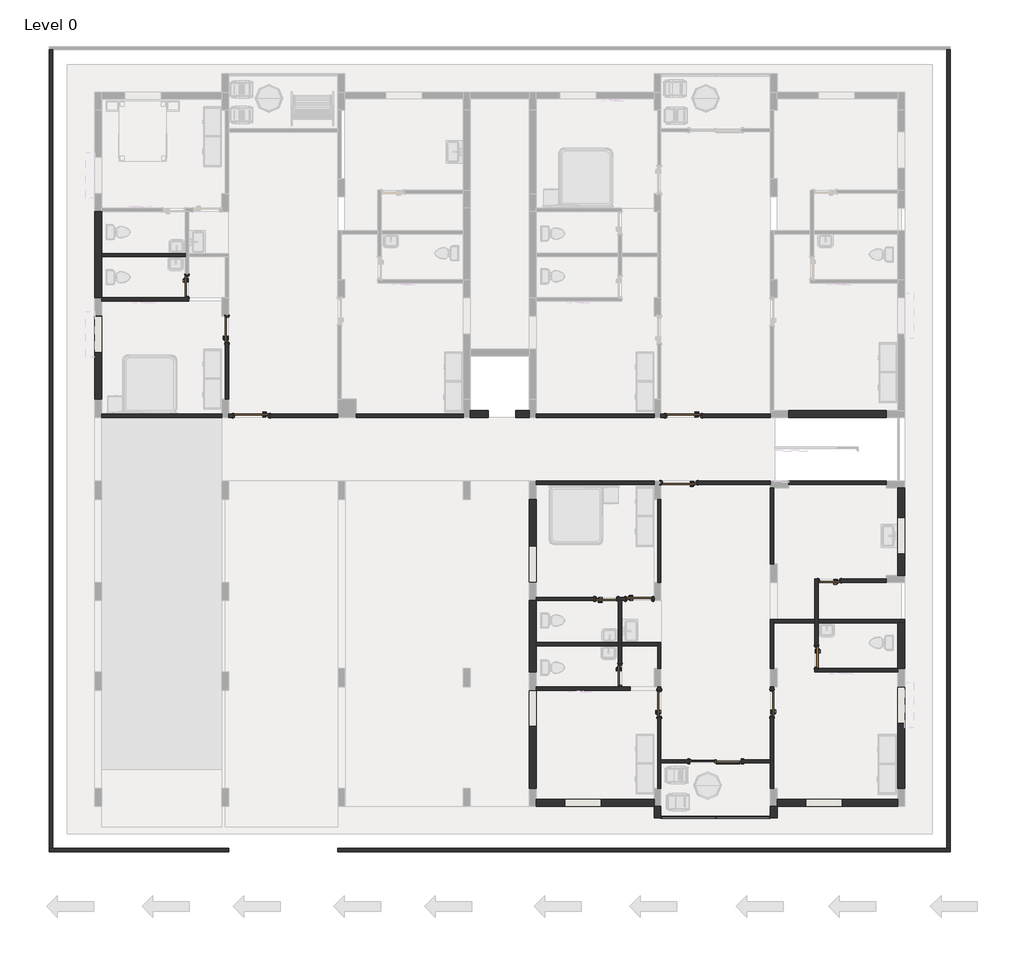
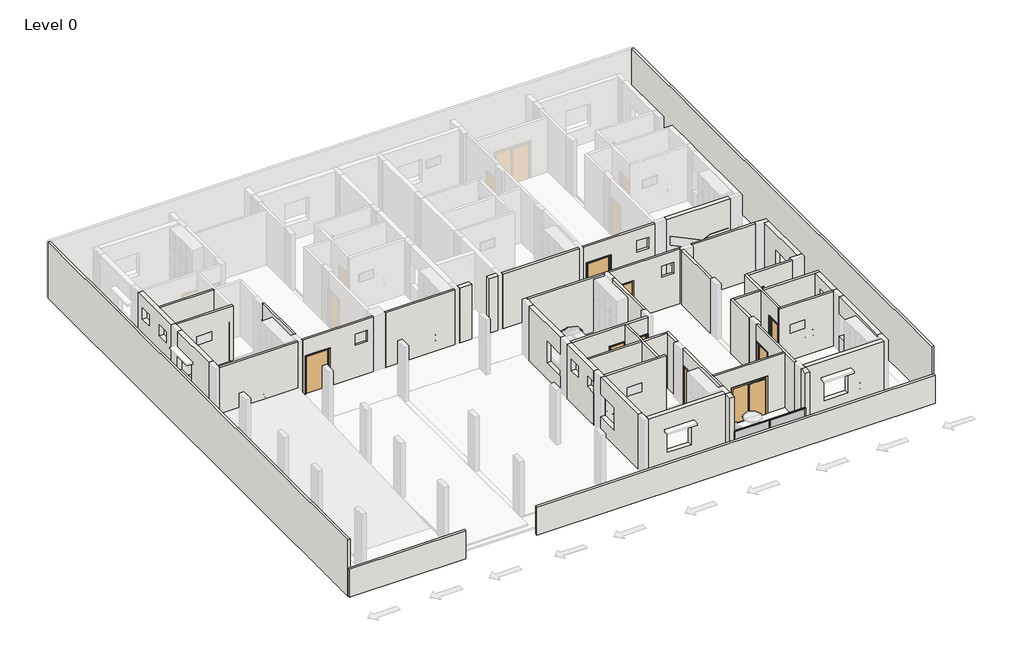
# One storey, part 1 of 6: 46 walls, 13 doors, 5 members, 2 plates.
"""IFC4 building model written with IfcOpenShell, lengths in millimetres."""

from ifc_helpers import new_model, si_unit, frame, origin, origin_with_axes, place, context, project, spatial, polyline, outline, extrude, faceted_brep, transform, mapped, element, save
from components import door_c5e969d5, door_d225582b, door_4bb05ab8, doors_intsgl_3_11801b65, doors_intsgl_3_f3216364, doors_intsgl_4_41b074ad, doors_intsgl_4_134d4d27, rectangular_mullion_30mm_square_b78902bc, rectangular_mullion_30mm_square_f98953c9, rectangular_mullion_30mm_square_8997babb, rectangular_mullion_30mm_square_5c6859bd, system_panel_glazed_e8634194, system_panel_glazed_30ab8f14

model = new_model("IFC4")

# Units and contexts
model_context = context("Model", 3, world=origin())
ifc_project = project(units=[si_unit("LENGTHUNIT", "METRE", prefix="MILLI")], contexts=[model_context])

# Site, building, storey
site = spatial("IfcSite", under=ifc_project)
building = spatial("IfcBuilding", under=site)
storey = spatial("IfcBuildingStorey", under=building, Name="Level 0", Elevation=0.0)

# Doors
placement = place(None, origin())
door_shape = door_c5e969d5(model_context)
element("IfcDoor", 1, ObjectType="Door-Double-Sliding : 5'8\"", at=placement, inside=storey, context=model_context, shape_type="MappedRepresentation", body=[
    mapped(door_shape, transform((7286.1098461, -11905.3017861, 0.0), x_axis=(-1.0, 0.0, 0.0), y_axis=(0.0, -1.0, 0.0), z_axis=(0.0, 0.0, 1.0))),
])
door_2_shape = door_d225582b(model_context)
element("IfcDoor", 2, ObjectType="Doors_IntSgl : 2'6\"", at=placement, inside=storey, context=model_context, shape_type="MappedRepresentation", body=[
    mapped(door_2_shape, transform((-10393.0197227, 3860.6022446, 0.0), x_axis=(0.0, -1.0, 0.0), y_axis=(1.0, 0.0, 0.0), z_axis=(0.0, 0.0, 1.0))),
])
element("IfcDoor", 3, ObjectType="Doors_IntSgl : 2'6\"", at=placement, inside=storey, context=model_context, shape_type="MappedRepresentation", body=[
    mapped(door_2_shape, transform((4085.7098461, -9155.7517861, 0.0), x_axis=(0.0, -1.0, 0.0), y_axis=(1.0, 0.0, 0.0), z_axis=(0.0, 0.0, 1.0))),
])
element("IfcDoor", 4, ObjectType="Doors_IntSgl : 2'6\"", at=placement, inside=storey, context=model_context, shape_type="MappedRepresentation", body=[
    mapped(door_2_shape, transform((3634.8598461, -6596.7017861, 0.0), x_axis=(1.0, 0.0, 0.0), y_axis=(0.0, 1.0, 0.0), z_axis=(0.0, 0.0, 1.0))),
])
door_3_shape = door_4bb05ab8(model_context)
element("IfcDoor", 5, ObjectType="Doors_IntSgl : 2'6\"", at=placement, inside=storey, context=model_context, shape_type="MappedRepresentation", body=[
    mapped(door_3_shape, transform((11096.1098461, -5987.1017861, 0.0), x_axis=(-1.0, 0.0, 0.0), y_axis=(0.0, -1.0, 0.0), z_axis=(0.0, 0.0, 1.0))),
])
element("IfcDoor", 6, ObjectType="Doors_IntSgl : 2'6\"", at=placement, inside=storey, context=model_context, shape_type="MappedRepresentation", body=[
    mapped(door_3_shape, transform((10657.9598461, -8546.1517861, 0.0), x_axis=(0.0, -1.0, 0.0), y_axis=(1.0, 0.0, 0.0), z_axis=(0.0, 0.0, 1.0))),
])
doors_intsgl_3_shape = doors_intsgl_3_11801b65(model_context)
element("IfcDoor", 7, ObjectType="Doors_IntSgl : 3'", at=placement, inside=storey, context=model_context, shape_type="MappedRepresentation", body=[
    mapped(doors_intsgl_3_shape, transform((-9058.7901539, 2413.9482139, 0.0), x_axis=(0.0, 1.0, 0.0), y_axis=(-1.0, 0.0, 0.0), z_axis=(0.0, 0.0, 1.0))),
])
element("IfcDoor", 8, ObjectType="Doors_IntSgl : 3'", at=placement, inside=storey, context=model_context, shape_type="MappedRepresentation", body=[
    mapped(doors_intsgl_3_shape, transform((5400.1598461, -10108.2517861, 0.0), x_axis=(0.0, 1.0, 0.0), y_axis=(-1.0, 0.0, 0.0), z_axis=(0.0, 0.0, 1.0))),
])
element("IfcDoor", 9, ObjectType="Doors_IntSgl : 3'", at=placement, inside=storey, context=model_context, shape_type="MappedRepresentation", body=[
    mapped(doors_intsgl_3_shape, transform((4733.4098461, -6596.7017861, 0.0), x_axis=(1.0, 0.0, 0.0), y_axis=(0.0, 1.0, 0.0), z_axis=(0.0, 0.0, 1.0))),
])
doors_intsgl_3_2_shape = doors_intsgl_3_f3216364(model_context)
element("IfcDoor", 10, ObjectType="Doors_IntSgl : 3'", at=placement, inside=storey, context=model_context, shape_type="MappedRepresentation", body=[
    mapped(doors_intsgl_3_2_shape, transform((9172.0598461, -10095.5517861, 0.0), x_axis=(0.0, 1.0, 0.0), y_axis=(-1.0, 0.0, 0.0), z_axis=(0.0, 0.0, 1.0))),
])
doors_intsgl_4_shape = doors_intsgl_4_41b074ad(model_context)
element("IfcDoor", 11, ObjectType="Doors_IntSgl : 4'", at=placement, inside=storey, context=model_context, shape_type="MappedRepresentation", body=[
    mapped(doors_intsgl_4_shape, transform((-8239.6401539, -463.7477554, 0.0), x_axis=(-1.0, 0.0, 0.0), y_axis=(0.0, -1.0, 0.0), z_axis=(0.0, 0.0, 1.0))),
])
element("IfcDoor", 12, ObjectType="Doors_IntSgl : 4'", at=placement, inside=storey, context=model_context, shape_type="MappedRepresentation", body=[
    mapped(doors_intsgl_4_shape, transform((6219.3098461, -462.6017861, 0.0), x_axis=(-1.0, 0.0, 0.0), y_axis=(0.0, -1.0, 0.0), z_axis=(0.0, 0.0, 1.0))),
])
doors_intsgl_4_2_shape = doors_intsgl_4_134d4d27(model_context)
element("IfcDoor", 13, ObjectType="Doors_IntSgl : 4'", at=placement, inside=storey, context=model_context, shape_type="MappedRepresentation", body=[
    mapped(doors_intsgl_4_2_shape, transform((6066.9098461, -2710.5017861, 0.0), x_axis=(-1.0, 0.0, 0.0), y_axis=(0.0, -1.0, 0.0), z_axis=(0.0, 0.0, 1.0))),
])

# Members
rectangular_mullion_30mm_square_shape = rectangular_mullion_30mm_square_b78902bc(model_context)
element("IfcMember", 14, ObjectType="Rectangular Mullion : 30mm_Square", at=placement, inside=storey, context=model_context, shape_type="MappedRepresentation", body=[
    mapped(rectangular_mullion_30mm_square_shape, transform((7272.9093803, -13918.2517861, 1164.8147652), x_axis=(0.0, 0.0, 1.0), y_axis=(0.0, -1.0, 0.0), z_axis=(1.0, 0.0, 0.0))),
])
rectangular_mullion_30mm_square_2_shape = rectangular_mullion_30mm_square_f98953c9(model_context)
element("IfcMember", 15, ObjectType="Rectangular Mullion : 30mm_Square", at=placement, inside=storey, context=model_context, shape_type="MappedRepresentation", body=[
    mapped(rectangular_mullion_30mm_square_2_shape, transform((9114.9098461, -13918.2517861, 98.0147652), x_axis=(1.0, 0.0, 0.0), y_axis=(0.0, -1.0, 0.0), z_axis=(0.0, 0.0, -1.0))),
])
rectangular_mullion_30mm_square_3_shape = rectangular_mullion_30mm_square_8997babb(model_context)
element("IfcMember", 16, ObjectType="Rectangular Mullion : 30mm_Square", at=placement, inside=storey, context=model_context, shape_type="MappedRepresentation", body=[
    mapped(rectangular_mullion_30mm_square_3_shape, transform((7287.9093803, -13918.2517861, 98.0147652), x_axis=(1.0, 0.0, 0.0), y_axis=(0.0, -1.0, 0.0), z_axis=(0.0, 0.0, -1.0))),
])
element("IfcMember", 17, ObjectType="Rectangular Mullion : 30mm_Square", at=placement, inside=storey, context=model_context, shape_type="MappedRepresentation", body=[
    mapped(rectangular_mullion_30mm_square_2_shape, transform((5457.90938, -13918.2517861, 1164.8147652), x_axis=(-1.0, 0.0, 0.0), y_axis=(0.0, -1.0, 0.0), z_axis=(0.0, 0.0, 1.0))),
])
rectangular_mullion_30mm_square_4_shape = rectangular_mullion_30mm_square_5c6859bd(model_context)
element("IfcMember", 18, ObjectType="Rectangular Mullion : 30mm_Square", at=placement, inside=storey, context=model_context, shape_type="MappedRepresentation", body=[
    mapped(rectangular_mullion_30mm_square_4_shape, transform((9084.9098461, -13918.2517861, 1164.8147652), x_axis=(0.0, 0.0, 1.0), y_axis=(0.0, -1.0, 0.0), z_axis=(1.0, 0.0, 0.0))),
])

# Plates
system_panel_glazed_shape = system_panel_glazed_e8634194(model_context)
element("IfcPlate", 19, ObjectType="System Panel : Glazed", at=placement, inside=storey, context=model_context, shape_type="MappedRepresentation", body=[
    mapped(system_panel_glazed_shape, transform((6372.9093801, -13918.2517861, 98.0147652), x_axis=(1.0, 0.0, 0.0), y_axis=(0.0, 1.0, 0.0), z_axis=(0.0, 0.0, 1.0))),
])
system_panel_glazed_2_shape = system_panel_glazed_30ab8f14(model_context)
element("IfcPlate", 20, ObjectType="System Panel : Glazed", at=placement, inside=storey, context=model_context, shape_type="MappedRepresentation", body=[
    mapped(system_panel_glazed_2_shape, transform((8201.4096132, -13918.2517861, 98.0147652), x_axis=(1.0, 0.0, 0.0), y_axis=(0.0, 1.0, 0.0), z_axis=(0.0, 0.0, 1.0))),
])

# Walls
element("IfcWall", 21, ObjectType="2\"", at=placement, inside=storey, context=model_context, shape_type="SweptSolid", body=[
    extrude(outline(polyline([(5457.90938, -13867.4517861), (9114.9098461, -13867.4517861), (9114.9098461, -13918.2517861), (5457.90938, -13918.2517861), (5457.90938, -13867.4517861)])), origin_with_axes(), (0.0, 0.0, 1.0), 98.0147652),
])
element("IfcWall", 22, ObjectType="9\"", at=placement, inside=storey, context=model_context, shape_type="SweptSolid", body=[
    extrude(outline(polyline([(13001.1098461, -291.1517861), (13001.1098461, -519.7517861), (9725.7585903, -519.7517861), (9725.7585903, -291.1517861), (13001.1098461, -291.1517861)])), origin_with_axes(), (0.0, 0.0, 1.0), 3048.0),
])
element("IfcWall", 23, ObjectType="9\"", at=placement, inside=storey, context=model_context, shape_type="SweptSolid", body=[
    extrude(outline(polyline([(-2881.9517861, 0.0), (-5815.6517861, 0.0), (-5815.6517861, 3048.0), (-2881.9517861, 3048.0), (-2881.9517861, 0.0)]), holes=[polyline([(-5092.3247708, 2133.6), (-5092.3247708, 914.4), (-3873.1247708, 914.4), (-3873.1247708, 2133.6), (-5092.3247708, 2133.6)])]), frame((13382.1098461, 0.0, 0.0), z_axis=(1.0, 0.0, 0.0), x_axis=(0.0, 1.0, 0.0)), (0.0, 0.0, 1.0), 228.6),
])
element("IfcWall", 24, ObjectType="9\"", at=placement, inside=storey, context=model_context, shape_type="SweptSolid", body=[
    extrude(outline(polyline([(-7403.1517861, 0.0), (-8927.1517861, 0.0), (-8927.1517861, 3048.0), (-7403.1517861, 3048.0), (-7403.1517861, 0.0)]), holes=[polyline([(-7860.3517861, 2438.4), (-8469.9517861, 2438.4), (-8469.9517861, 1828.8), (-7860.3517861, 1828.8), (-7860.3517861, 2438.4)])]), frame((13382.1098461, 0.0, 0.0), z_axis=(1.0, 0.0, 0.0), x_axis=(0.0, 1.0, 0.0)), (0.0, 0.0, 1.0), 228.6),
])
element("IfcWall", 25, ObjectType="9\"", at=placement, inside=storey, context=model_context, shape_type="SweptSolid", body=[
    extrude(outline(polyline([(-9536.7517861, 914.4), (-9536.7517861, 0.0), (-12927.6517861, 0.0), (-12927.6517861, 3048.0), (-9536.7517861, 3048.0), (-9536.7517861, 2133.6), (-10755.9517861, 2133.6), (-10755.9517861, 914.4), (-9536.7517861, 914.4)])), frame((13382.1098461, 0.0, 0.0), z_axis=(1.0, 0.0, 0.0), x_axis=(0.0, 1.0, 0.0)), (0.0, 0.0, 1.0), 228.6),
])
element("IfcWall", 26, ObjectType="9\"", at=placement, inside=storey, context=model_context, shape_type="SweptSolid", body=[
    extrude(outline(polyline([(0.0, 13382.1098461), (3048.0, 13382.1098461), (3048.0, 9343.4965978), (0.0, 9343.4965978), (0.0, 13382.1098461)]), holes=[polyline([(2133.6, 10294.7737348), (2133.6, 11513.9737348), (914.4, 11513.9737348), (914.4, 10294.7737348), (2133.6, 10294.7737348)])]), frame((0.0, -13537.2517861, 0.0), z_axis=(0.0, 1.0, 0.0), x_axis=(0.0, 0.0, 1.0)), (0.0, 0.0, 1.0), 228.6),
])
element("IfcWall", 27, ObjectType="9\"", at=placement, inside=storey, context=model_context, shape_type="Brep", body=[
    faceted_brep([(9114.9098461, -13537.2517861, 0.0), (9114.9098461, -13867.4517861, 0.0), (9114.9098461, -13918.2517861, 0.0), (9114.9098461, -13918.2517861, 98.0147652), (9114.9098461, -13918.2517861, 3048.0), (9114.9098461, -13537.2517861, 3048.0), (9343.5098461, -13537.2517861, 0.0), (9343.5098461, -13537.2517861, 3048.0), (9343.5098461, -13918.2517861, 3048.0), (9343.5098461, -13918.2517861, 0.0)], [[[0, 1, 2, 3, 4, 5]], [[6, 7, 8, 9]], [[2, 1, 0, 6, 9]], [[4, 3, 2, 9, 8]], [[5, 4, 8, 7]], [[0, 5, 7, 6]]]),
])
element("IfcWall", 28, ObjectType="9\"", at=placement, inside=storey, context=model_context, shape_type="Brep", body=[
    faceted_brep([(5229.30938, -13537.2517861, 0.0), (5229.30938, -13918.2517861, 0.0), (5229.30938, -13918.2517861, 3048.0), (5229.30938, -13537.2517861, 3048.0), (5457.90938, -13537.2517861, 0.0), (5457.90938, -13537.2517861, 3048.0), (5457.90938, -13918.2517861, 3048.0), (5457.90938, -13918.2517861, 98.0147652), (5457.90938, -13918.2517861, 0.0), (5457.90938, -13867.4517861, 0.0)], [[[0, 1, 2, 3]], [[4, 5, 6, 7, 8, 9]], [[1, 0, 4, 9, 8]], [[2, 1, 8, 7, 6]], [[3, 2, 6, 5]], [[0, 3, 5, 4]]]),
])
element("IfcWall", 29, ObjectType="9\"", at=placement, inside=storey, context=model_context, shape_type="SweptSolid", body=[
    extrude(outline(polyline([(0.0, 1285.3598461), (0.0, 5229.30938), (3048.0, 5229.30938), (3048.0, 1285.3598461), (0.0, 1285.3598461)]), holes=[polyline([(2133.6, 3455.8237348), (914.4, 3455.8237348), (914.4, 2236.6237348), (2133.6, 2236.6237348), (2133.6, 3455.8237348)])]), frame((0.0, -13537.2517861, 0.0), z_axis=(0.0, 1.0, 0.0), x_axis=(0.0, 0.0, 1.0)), (0.0, 0.0, 1.0), 228.6),
])
element("IfcWall", 30, ObjectType="9\"", at=placement, inside=storey, context=model_context, shape_type="SweptSolid", body=[
    extrude(outline(polyline([(-9651.0517861, 0.0), (-12927.6517861, 0.0), (-12927.6517861, 3048.0), (-9651.0517861, 3048.0), (-9651.0517861, 2133.6), (-10870.2517861, 2133.6), (-10870.2517861, 914.4), (-9651.0517861, 914.4), (-9651.0517861, 0.0)])), frame((1056.7598461, 0.0, 0.0), z_axis=(1.0, 0.0, 0.0), x_axis=(0.0, 1.0, 0.0)), (0.0, 0.0, 1.0), 228.6),
])
element("IfcWall", 31, ObjectType="9\"", at=placement, inside=storey, context=model_context, shape_type="SweptSolid", body=[
    extrude(outline(polyline([(-8431.8517861, 2438.4), (-9041.4517861, 2438.4), (-9041.4517861, 3048.0), (-6653.8517861, 3048.0), (-6653.8517861, 0.0), (-9041.4517861, 0.0), (-9041.4517861, 1828.8), (-8431.8517861, 1828.8), (-8431.8517861, 2438.4)]), holes=[polyline([(-7032.3347219, 2438.4), (-7641.9347219, 2438.4), (-7641.9347219, 1828.8), (-7032.3347219, 1828.8), (-7032.3347219, 2438.4)])]), frame((1056.7598461, 0.0, 0.0), z_axis=(1.0, 0.0, 0.0), x_axis=(0.0, 1.0, 0.0)), (0.0, 0.0, 1.0), 228.6),
])
element("IfcWall", 32, ObjectType="9\"", at=placement, inside=storey, context=model_context, shape_type="SweptSolid", body=[
    extrude(outline(polyline([(-4825.0517861, 2133.6), (-6044.2517861, 2133.6), (-6044.2517861, 3048.0), (-3262.9517861, 3048.0), (-3262.9517861, 0.0), (-6044.2517861, 0.0), (-6044.2517861, 914.4), (-4825.0517861, 914.4), (-4825.0517861, 2133.6)])), frame((1056.7598461, 0.0, 0.0), z_axis=(1.0, 0.0, 0.0), x_axis=(0.0, 1.0, 0.0)), (0.0, 0.0, 1.0), 228.6),
])
element("IfcWall", 33, ObjectType="9\"", at=placement, inside=storey, context=model_context, shape_type="SweptSolid", body=[
    extrude(outline(polyline([(6362.5022446, 0.0), (3480.7482139, 0.0), (3480.7482139, 3048.0), (6362.5022446, 3048.0), (6362.5022446, 0.0)]), holes=[polyline([(4473.8652782, 2438.4), (3864.2652782, 2438.4), (3864.2652782, 1828.8), (4473.8652782, 1828.8), (4473.8652782, 2438.4)]), polyline([(5984.0193089, 2438.4), (5374.4193089, 2438.4), (5374.4193089, 1828.8), (5984.0193089, 1828.8), (5984.0193089, 2438.4)])]), frame((-13478.3901539, 0.0, 0.0), z_axis=(1.0, 0.0, 0.0), x_axis=(0.0, 1.0, 0.0)), (0.0, 0.0, 1.0), 228.6),
])
element("IfcWall", 34, ObjectType="9\"", at=placement, inside=storey, context=model_context, shape_type="SweptSolid", body=[
    extrude(outline(polyline([(2871.1482139, 3048.0), (2871.1482139, 0.0), (89.8788513, 0.0), (89.8788513, 3048.0), (2871.1482139, 3048.0)]), holes=[polyline([(1650.8022446, 914.4), (2870.0022446, 914.4), (2870.0022446, 2133.6), (1650.8022446, 2133.6), (1650.8022446, 914.4)])]), frame((-13478.3901539, 0.0, 0.0), z_axis=(1.0, 0.0, 0.0), x_axis=(0.0, 1.0, 0.0)), (0.0, 0.0, 1.0), 228.6),
])
element("IfcWall", 35, ObjectType="9\"", at=placement, inside=storey, context=model_context, shape_type="SweptSolid", body=[
    extrude(outline(polyline([(-314.8400495, -519.7517861), (-924.4401539, -519.7517861), (-924.4401539, -291.1517861), (-314.8400495, -291.1517861), (-314.8400495, -519.7517861)])), origin_with_axes(), (0.0, 0.0, 1.0), 3048.0),
])
element("IfcWall", 36, ObjectType="9\"", at=placement, inside=storey, context=model_context, shape_type="SweptSolid", body=[
    extrude(outline(polyline([(1056.7598461, -519.7517862), (599.5599505, -519.7517861), (599.5599505, -291.1517861), (1056.7598461, -291.1517862), (1056.7598461, -519.7517862)])), origin_with_axes(), (0.0, 0.0, 1.0), 3048.0),
])
element("IfcWall", 37, ObjectType="Brick Wall 4.5\"", at=placement, inside=storey, context=model_context, shape_type="SweptSolid", body=[
    extrude(outline(polyline([(-10449.4401539, 4851.2022446), (-13249.7901539, 4851.2022446), (-13249.7901539, 4965.5022446), (-10449.4401539, 4965.5022446), (-10449.4401539, 4851.2022446)])), origin_with_axes(), (0.0, 0.0, 1.0), 3048.0),
])
element("IfcWall", 38, ObjectType="Brick Wall 4.5\"", at=placement, inside=storey, context=model_context, shape_type="SweptSolid", body=[
    extrude(outline(polyline([(88.7022446, 3048.0), (2871.1482139, 3048.0), (2871.1482139, 2133.6), (1956.7482139, 2133.6), (1956.7482139, 0.0), (88.7022446, 0.0), (88.7022446, 3048.0)])), frame((-9115.9401539, 0.0, 0.0), z_axis=(1.0, 0.0, 0.0), x_axis=(0.0, 1.0, 0.0)), (0.0, 0.0, 1.0), 114.3),
])
element("IfcWall", 39, ObjectType="Brick Wall 4.5\"", at=placement, inside=storey, context=model_context, shape_type="SweptSolid", body=[
    extrude(outline(polyline([(3048.0, -9001.6401539), (0.0, -9001.6401539), (0.0, -8849.2401539), (2133.6, -8849.2401539), (2133.6, -7630.0401539), (0.0, -7630.0401539), (0.0, -5344.0401539), (3048.0, -5344.0401539), (3048.0, -9001.6401539)]), holes=[polyline([(2438.4, -5671.4887701), (1828.8, -5671.4887701), (1828.8, -6281.0887701), (2438.4, -6281.0887701), (2438.4, -5671.4887701)])]), frame((0.0, -520.8977554, 0.0), z_axis=(0.0, 1.0, 0.0), x_axis=(0.0, 0.0, 1.0)), (0.0, 0.0, 1.0), 114.3),
])
element("IfcWall", 40, ObjectType="Brick Wall 4.5\"", at=placement, inside=storey, context=model_context, shape_type="SweptSolid", body=[
    extrude(outline(polyline([(-13249.7901539, -406.5977554), (-9230.2401539, -406.5977554), (-9230.2401539, -520.8977554), (-13249.7901539, -520.8977554), (-13249.7901539, -406.5977554)])), origin_with_axes(), (0.0, 0.0, 1.0), 3048.0),
])
element("IfcWall", 41, ObjectType="Brick Wall 4.5\"", at=placement, inside=storey, context=model_context, shape_type="Brep", body=[
    faceted_brep([(-10335.1401539, 3479.6022446, 0.0), (-13249.7901539, 3479.6022446, 0.0), (-13249.7901539, 3479.6022446, 3048.0), (-10450.1697227, 3479.6022446, 3048.0), (-10335.8697227, 3479.6022446, 3048.0), (-10335.1401539, 3479.6022446, 3048.0), (-10335.1401539, 3365.3022446, 0.0), (-10335.1401539, 3365.3022446, 3048.0), (-13249.7901539, 3365.3022446, 3048.0), (-13249.7901539, 3365.3022446, 0.0)], [[[0, 1, 2, 3, 4, 5]], [[6, 7, 8, 9]], [[1, 0, 6, 9]], [[2, 1, 9, 8]], [[5, 4, 3, 2, 8, 7]], [[0, 5, 7, 6]]]),
])
element("IfcWall", 42, ObjectType="Brick Wall 4.5\"", at=placement, inside=storey, context=model_context, shape_type="SweptSolid", body=[
    extrude(outline(polyline([(3048.0, 5457.3098461), (0.0, 5457.3098461), (0.0, 5609.7098461), (2133.6, 5609.7098461), (2133.6, 6828.9098461), (0.0, 6828.9098461), (0.0, 9114.9098461), (3048.0, 9114.9098461), (3048.0, 5457.3098461)]), holes=[polyline([(2438.4, 8177.8612299), (2438.4, 8787.4612299), (1828.8, 8787.4612299), (1828.8, 8177.8612299), (2438.4, 8177.8612299)])]), frame((0.0, -519.7517861, 0.0), z_axis=(0.0, 1.0, 0.0), x_axis=(0.0, 0.0, 1.0)), (0.0, 0.0, 1.0), 114.3),
])
element("IfcWall", 43, ObjectType="Brick Wall 4.5\"", at=placement, inside=storey, context=model_context, shape_type="SweptSolid", body=[
    extrude(outline(polyline([(1285.3598461, -405.4517861), (5228.7098461, -405.4517861), (5228.7098461, -519.7517861), (1285.3598461, -519.7517861), (1285.3598461, -405.4517861)])), origin_with_axes(), (0.0, 0.0, 1.0), 3048.0),
])
element("IfcWall", 44, ObjectType="Brick Wall 4.5\"", at=placement, inside=storey, context=model_context, shape_type="SweptSolid", body=[
    extrude(outline(polyline([(-4734.4401539, -406.5977554), (-1153.0401539, -406.5977554), (-1153.0401539, -520.8977554), (-4734.4401539, -520.8977554), (-4734.4401539, -406.5977554)])), origin_with_axes(), (0.0, 0.0, 1.0), 3048.0),
])
element("IfcWall", 45, ObjectType="Brick Wall 4.5\"", at=placement, inside=storey, context=model_context, shape_type="SweptSolid", body=[
    extrude(outline(polyline([(5228.7098461, -2767.0150775), (1285.3598461, -2767.0150775), (1285.3598461, -2652.7150775), (5228.7098461, -2652.7150775), (5228.7098461, -2767.0150775)])), origin_with_axes(), (0.0, 0.0, 1.0), 3048.0),
])
element("IfcWall", 46, ObjectType="Brick Wall 4.5\"", at=placement, inside=storey, context=model_context, shape_type="SweptSolid", body=[
    extrude(outline(polyline([(5457.3098461, -3262.9517861), (5457.3098461, -6044.2517861), (5343.0098461, -6044.2517861), (5343.0098461, -3262.9517861), (5457.3098461, -3262.9517861)])), origin_with_axes(), (0.0, 0.0, 1.0), 3048.0),
])
element("IfcWall", 47, ObjectType="Brick Wall 4.5\"", at=placement, inside=storey, context=model_context, shape_type="SweptSolid", body=[
    extrude(outline(polyline([(0.0, 9114.9098461), (3048.0, 9114.9098461), (3048.0, 5457.3098461), (2133.6, 5457.3098461), (2133.6, 6676.5098461), (0.0, 6676.5098461), (0.0, 9114.9098461)]), holes=[polyline([(2438.4, 8787.4612299), (1828.8, 8787.4612299), (1828.8, 8177.8612299), (2438.4, 8177.8612299), (2438.4, 8787.4612299)])]), frame((0.0, -2767.6517861, 0.0), z_axis=(0.0, 1.0, 0.0), x_axis=(0.0, 0.0, 1.0)), (0.0, 0.0, 1.0), 114.3),
])
element("IfcWall", 48, ObjectType="Brick Wall 4.5\"", at=placement, inside=storey, context=model_context, shape_type="SweptSolid", body=[
    extrude(outline(polyline([(9229.2098461, -2881.9517861), (9229.2098461, -5434.6517861), (9114.9098461, -5434.6517861), (9114.9098461, -2881.9517861), (9229.2098461, -2881.9517861)])), origin_with_axes(), (0.0, 0.0, 1.0), 3048.0),
])
element("IfcWall", 49, ObjectType="Brick Wall 4.5\"", at=placement, inside=storey, context=model_context, shape_type="SweptSolid", body=[
    extrude(outline(polyline([(13001.1098461, -2767.6517861), (9724.5098461, -2767.6517861), (9724.5098461, -2653.3517861), (13001.1098461, -2653.3517861), (13001.1098461, -2767.6517861)])), origin_with_axes(), (0.0, 0.0, 1.0), 3048.0),
])
element("IfcWall", 50, ObjectType="Brick Wall 4.5\"", at=placement, inside=storey, context=model_context, shape_type="SweptSolid", body=[
    extrude(outline(polyline([(3048.0, 13001.1098461), (3048.0, 10715.1098461), (2133.6, 10715.1098461), (2133.6, 11477.1098461), (0.0, 11477.1098461), (0.0, 13001.1098461), (3048.0, 13001.1098461)])), frame((0.0, -6044.2517861, 0.0), z_axis=(0.0, 1.0, 0.0), x_axis=(0.0, 0.0, 1.0)), (0.0, 0.0, 1.0), 114.3),
])
element("IfcWall", 51, ObjectType="Brick Wall 4.5\"", at=placement, inside=storey, context=model_context, shape_type="Brep", body=[
    faceted_brep([(10715.1098461, -5929.9517861, 0.0), (10715.1098461, -5929.9517861, 2133.6), (10715.1098461, -5929.9517861, 3048.0), (10715.1098461, -6044.2517861, 3048.0), (10715.1098461, -7288.8517861, 3048.0), (10715.1098461, -7403.1517861, 3048.0), (10715.1098461, -8927.1517861, 3048.0), (10715.1098461, -8927.1517861, 2133.6), (10715.1098461, -8165.1517861, 2133.6), (10715.1098461, -8165.1517861, 0.0), (10715.1098461, -7403.1517861, 0.0), (10715.1098461, -7288.8517861, 0.0), (10600.8098461, -5929.9517861, 3048.0), (10600.8098461, -5929.9517861, 0.0), (10600.8098461, -7288.8517861, 0.0), (10600.8098461, -7403.1517861, 0.0), (10600.8098461, -8165.1517861, 0.0), (10600.8098461, -8165.1517861, 2133.6), (10600.8098461, -8927.1517861, 2133.6), (10600.8098461, -8927.1517861, 3048.0), (10600.8098461, -7403.1517861, 3048.0), (10600.8098461, -7288.8517861, 3048.0)], [[[0, 1, 2, 3, 4, 5, 6, 7, 8, 9, 10, 11]], [[12, 13, 14, 15, 16, 17, 18, 19, 20, 21]], [[13, 0, 11, 10, 9, 16, 15, 14]], [[2, 1, 0, 13, 12]], [[6, 5, 4, 3, 2, 12, 21, 20, 19]], [[6, 19, 18, 7]], [[17, 8, 7, 18]], [[8, 17, 16, 9]]]),
])
element("IfcWall", 52, ObjectType="Brick Wall 4.5\"", at=placement, inside=storey, context=model_context, shape_type="SweptSolid", body=[
    extrude(outline(polyline([(13610.7098461, -7288.8517861), (13610.7098461, -7403.1517861), (10715.1098461, -7403.1517861), (10715.1098461, -7288.8517861), (13610.7098461, -7288.8517861)])), origin_with_axes(), (0.0, 0.0, 1.0), 3048.0),
    extrude(outline(polyline([(9229.2098461, -7403.1517861), (9229.2098461, -7288.8517861), (10600.8098461, -7288.8517861), (10600.8098461, -7403.1517861), (9229.2098461, -7403.1517861)])), origin_with_axes(), (0.0, 0.0, 1.0), 3048.0),
])
element("IfcWall", 53, ObjectType="Brick Wall 4.5\"", at=placement, inside=storey, context=model_context, shape_type="Brep", body=[
    faceted_brep([(9229.2098461, -8927.1517861, 0.0), (9229.2098461, -7403.1517861, 0.0), (9229.2098461, -7288.8517861, 0.0), (9229.2098461, -7288.8517861, 3048.0), (9229.2098461, -7403.1517861, 3048.0), (9229.2098461, -8927.1517861, 3048.0), (9114.9098461, -8927.1517861, 0.0), (9114.9098461, -8927.1517861, 3048.0), (9114.9098461, -7288.8517861, 3048.0), (9114.9098461, -7288.8517861, 0.0)], [[[0, 1, 2, 3, 4, 5]], [[6, 7, 8, 9]], [[2, 1, 0, 6, 9]], [[3, 2, 9, 8]], [[5, 4, 3, 8, 7]], [[0, 5, 7, 6]]]),
])
element("IfcWall", 54, ObjectType="Brick Wall 4.5\"", at=placement, inside=storey, context=model_context, shape_type="Brep", body=[
    faceted_brep([(10600.8098461, -9041.4517861, 0.0), (13382.1098461, -9041.4517861, 0.0), (13382.1098461, -9041.4517861, 3048.0), (10600.8098461, -9041.4517861, 3048.0), (10600.8098461, -8927.1517861, 0.0), (10600.8098461, -8927.1517861, 2133.6), (10600.8098461, -8927.1517861, 3048.0), (10715.1098461, -8927.1517861, 3048.0), (13382.1098461, -8927.1517861, 3048.0), (13382.1098461, -8927.1517861, 0.0)], [[[0, 1, 2, 3]], [[4, 5, 6, 7, 8, 9]], [[1, 0, 4, 9]], [[2, 1, 9, 8]], [[3, 2, 8, 7, 6]], [[0, 3, 6, 5, 4]]]),
])
element("IfcWall", 55, ObjectType="Brick Wall 4.5\"", at=placement, inside=storey, context=model_context, shape_type="SweptSolid", body=[
    extrude(outline(polyline([(-9536.7517861, 3048.0), (-9536.7517861, 0.0), (-9638.3517861, 0.0), (-9638.3517861, 2133.6), (-10552.7517861, 2133.6), (-10552.7517861, 0.0), (-12927.6517861, 0.0), (-12927.6517861, 3048.0), (-9536.7517861, 3048.0)])), frame((9114.9098461, 0.0, 0.0), z_axis=(1.0, 0.0, 0.0), x_axis=(0.0, 1.0, 0.0)), (0.0, 0.0, 1.0), 114.3),
])
element("IfcWall", 56, ObjectType="Brick Wall 4.5\"", at=placement, inside=storey, context=model_context, shape_type="SweptSolid", body=[
    extrude(outline(polyline([(0.0, 5457.3098461), (0.0, 6422.5098461), (2032.0, 6422.5098461), (2032.0, 8149.7098461), (0.0, 8149.7098461), (0.0, 9114.9098461), (3048.0, 9114.9098461), (3048.0, 5457.3098461), (0.0, 5457.3098461)])), frame((0.0, -12089.4517861, 0.0), z_axis=(0.0, 1.0, 0.0), x_axis=(0.0, 0.0, 1.0)), (0.0, 0.0, 1.0), 114.3),
])
element("IfcWall", 57, ObjectType="Brick Wall 4.5\"", at=placement, inside=storey, context=model_context, shape_type="Brep", body=[
    faceted_brep([(5457.3098461, -9536.7517861, 0.0), (5457.3098461, -9536.7517861, 3048.0), (5457.3098461, -11975.1517861, 3048.0), (5457.3098461, -12089.4517861, 3048.0), (5457.3098461, -12927.6517861, 3048.0), (5457.3098461, -12927.6517861, 0.0), (5457.3098461, -12089.4517861, 0.0), (5457.3098461, -11975.1517861, 0.0), (5457.3098461, -10565.4517861, 0.0), (5457.3098461, -10565.4517861, 2133.6), (5457.3098461, -9651.0517861, 2133.6), (5457.3098461, -9651.0517861, 0.0), (5343.0098461, -9536.7517861, 3048.0), (5343.0098461, -9536.7517861, 0.0), (5343.0098461, -9651.0517861, 0.0), (5343.0098461, -9651.0517861, 2133.6), (5343.0098461, -10565.4517861, 2133.6), (5343.0098461, -10565.4517861, 0.0), (5343.0098461, -12927.6517861, 0.0), (5343.0098461, -12927.6517861, 3048.0)], [[[0, 1, 2, 3, 4, 5, 6, 7, 8, 9, 10, 11]], [[12, 13, 14, 15, 16, 17, 18, 19]], [[13, 0, 11, 14]], [[5, 18, 17, 8, 7, 6]], [[1, 0, 13, 12]], [[4, 3, 2, 1, 12, 19]], [[5, 4, 19, 18]], [[10, 15, 14, 11]], [[15, 10, 9, 16]], [[16, 9, 8, 17]]]),
])
element("IfcWall", 58, ObjectType="Brick Wall 4.5\"", at=placement, inside=storey, context=model_context, shape_type="Brep", body=[
    faceted_brep([(1285.3598461, -9651.0517861, 0.0), (4428.2038363, -9651.0517861, 0.0), (4428.2038363, -9651.0517861, 3048.0), (1285.3598461, -9651.0517861, 3048.0), (1285.3598461, -9536.7517861, 0.0), (1285.3598461, -9536.7517861, 3048.0), (4028.5598461, -9536.7517861, 3048.0), (4142.8598461, -9536.7517861, 3048.0), (4428.2038363, -9536.7517861, 3048.0), (4428.2038363, -9536.7517861, 0.0)], [[[0, 1, 2, 3]], [[4, 5, 6, 7, 8, 9]], [[1, 0, 4, 9]], [[2, 1, 9, 8]], [[3, 2, 8, 7, 6, 5]], [[0, 3, 5, 4]]]),
])
element("IfcWall", 59, ObjectType="Brick Wall 4.5\"", at=placement, inside=storey, context=model_context, shape_type="Brep", body=[
    faceted_brep([(4142.8598461, -6653.8517861, 0.0), (4142.8598461, -6653.8517861, 3048.0), (4142.8598461, -8050.8517861, 3048.0), (4142.8598461, -8165.1517861, 3048.0), (4142.8598461, -9536.7517861, 3048.0), (4142.8598461, -9536.7517861, 2133.6), (4142.8598461, -8774.7517861, 2133.6), (4142.8598461, -8774.7517861, 0.0), (4142.8598461, -8165.1517861, 0.0), (4142.8598461, -8050.8517861, 0.0), (4028.5598461, -6653.8517861, 3048.0), (4028.5598461, -6653.8517861, 0.0), (4028.5598461, -8050.8517861, 0.0), (4028.5598461, -8165.1517861, 0.0), (4028.5598461, -8774.7517861, 0.0), (4028.5598461, -8774.7517861, 2133.6), (4028.5598461, -9536.7517861, 2133.6), (4028.5598461, -9536.7517861, 3048.0), (4028.5598461, -8165.1517861, 3048.0), (4028.5598461, -8050.8517861, 3048.0)], [[[0, 1, 2, 3, 4, 5, 6, 7, 8, 9]], [[10, 11, 12, 13, 14, 15, 16, 17, 18, 19]], [[11, 0, 9, 8, 7, 14, 13, 12]], [[1, 0, 11, 10]], [[4, 3, 2, 1, 10, 19, 18, 17]], [[4, 17, 16, 5]], [[15, 6, 5, 16]], [[6, 15, 14, 7]]]),
])
element("IfcWall", 60, ObjectType="Brick Wall 4.5\"", at=placement, inside=storey, context=model_context, shape_type="SweptSolid", body=[
    extrude(outline(polyline([(5343.0098461, -8050.8517861), (5343.0098461, -8165.1517861), (4142.8598461, -8165.1517861), (4142.8598461, -8050.8517861), (5343.0098461, -8050.8517861)])), origin_with_axes(), (0.0, 0.0, 1.0), 3048.0),
    extrude(outline(polyline([(1285.3598461, -8165.1517861), (1285.3598461, -8050.8517861), (4028.5598461, -8050.8517861), (4028.5598461, -8165.1517861), (1285.3598461, -8165.1517861)])), origin_with_axes(), (0.0, 0.0, 1.0), 3048.0),
])
element("IfcWall", 61, ObjectType="Brick Wall 4.5\"", at=placement, inside=storey, context=model_context, shape_type="Brep", body=[
    faceted_brep([(5228.7098461, -6653.8517861, 0.0), (5228.7098461, -6653.8517861, 3048.0), (4142.8598461, -6653.8517861, 3048.0), (4028.5598461, -6653.8517861, 3048.0), (1285.3598461, -6653.8517861, 3048.0), (1285.3598461, -6653.8517861, 0.0), (3253.8598461, -6653.8517861, 0.0), (3253.8598461, -6653.8517861, 2133.6), (4015.8598461, -6653.8517861, 2133.6), (4015.8598461, -6653.8517861, 0.0), (4028.5598461, -6653.8517861, 0.0), (4142.8598461, -6653.8517861, 0.0), (4276.2098461, -6653.8517861, 0.0), (4276.2098461, -6653.8517861, 2133.6), (5190.6098461, -6653.8517861, 2133.6), (5190.6098461, -6653.8517861, 0.0), (5228.7098461, -6539.5517861, 3048.0), (5228.7098461, -6539.5517861, 0.0), (5190.6098461, -6539.5517861, 0.0), (5190.6098461, -6539.5517861, 2133.6), (4276.2098461, -6539.5517861, 2133.6), (4276.2098461, -6539.5517861, 0.0), (4015.8598461, -6539.5517861, 0.0), (4015.8598461, -6539.5517861, 2133.6), (3253.8598461, -6539.5517861, 2133.6), (3253.8598461, -6539.5517861, 0.0), (1285.3598461, -6539.5517861, 0.0), (1285.3598461, -6539.5517861, 3048.0)], [[[0, 1, 2, 3, 4, 5, 6, 7, 8, 9, 10, 11, 12, 13, 14, 15]], [[16, 17, 18, 19, 20, 21, 22, 23, 24, 25, 26, 27]], [[17, 0, 15, 18]], [[5, 26, 25, 6]], [[9, 22, 21, 12, 11, 10]], [[1, 0, 17, 16]], [[4, 3, 2, 1, 16, 27]], [[5, 4, 27, 26]], [[8, 23, 22, 9]], [[23, 8, 7, 24]], [[24, 7, 6, 25]], [[14, 19, 18, 15]], [[19, 14, 13, 20]], [[20, 13, 12, 21]]]),
])
element("IfcWall", 62, ObjectType="Brick Wall 4.5\"", at=placement, inside=storey, context=model_context, shape_type="Brep", body=[
    faceted_brep([(5457.3098461, -8927.1517861, 0.0), (5457.3098461, -8050.8517861, 0.0), (5457.3098461, -8050.8517861, 3048.0), (5457.3098461, -8927.1517861, 3048.0), (5343.0098461, -8927.1517861, 0.0), (5343.0098461, -8927.1517861, 3048.0), (5343.0098461, -8165.1517861, 3048.0), (5343.0098461, -8050.8517861, 3048.0), (5343.0098461, -8050.8517861, 0.0), (5343.0098461, -8165.1517861, 0.0)], [[[0, 1, 2, 3]], [[4, 5, 6, 7, 8, 9]], [[1, 0, 4, 9, 8]], [[2, 1, 8, 7]], [[3, 2, 7, 6, 5]], [[0, 3, 5, 4]]]),
])
element("IfcWall", 63, ObjectType="Shear Wall 4.5\" 2", at=placement, inside=storey, context=model_context, shape_type="Brep", body=[
    faceted_brep([(-14888.0901539, -14946.9517861, 0.0), (-14888.0901539, 11773.8482139, 0.0), (-14888.0901539, 11773.8482139, 3048.0), (-14888.0901539, -14946.9517861, 3048.0), (-15002.3901539, -14946.9517861, 0.0), (-15002.3901539, -14946.9517861, 1524.0), (-15002.3901539, -14946.9517861, 3048.0), (-15002.3901539, 11773.8482139, 3048.0), (-15002.3901539, 11773.8482139, 0.0)], [[[0, 1, 2, 3]], [[4, 5, 6, 7, 8]], [[1, 0, 4, 8]], [[2, 1, 8, 7]], [[3, 2, 7, 6]], [[0, 3, 6, 5, 4]]]),
])
element("IfcWall", 64, ObjectType="Shear Wall 4.5\" 2", at=placement, inside=storey, context=model_context, shape_type="Brep", body=[
    faceted_brep([(15134.7098461, -14946.9517861, 0.0), (15134.7098461, 11773.8482139, 0.0), (15134.7098461, 11773.8482139, 3048.0), (15134.7098461, -14946.9517861, 3048.0), (15134.7098461, -14946.9517861, 1524.0), (15020.4098461, -14946.9517861, 0.0), (15020.4098461, -14946.9517861, 3048.0), (15020.4098461, 11773.8482139, 3048.0), (15020.4098461, 11773.8482139, 0.0)], [[[0, 1, 2, 3, 4]], [[5, 6, 7, 8]], [[1, 0, 5, 8]], [[2, 1, 8, 7]], [[3, 2, 7, 6]], [[0, 4, 3, 6, 5]]]),
])
element("IfcWall", 65, ObjectType="Shear Wall 4.5\" 2", at=placement, inside=storey, context=model_context, shape_type="Brep", body=[
    faceted_brep([(-15002.3901539, -15061.2517861, 0.0), (-9001.6401539, -15061.2517861, 0.0), (-9001.6401539, -15061.2517861, 1524.0), (-15002.3901539, -15061.2517861, 1524.0), (-15002.3901539, -14946.9517861, 0.0), (-15002.3901539, -14946.9517861, 1524.0), (-9001.6401539, -14946.9517861, 1524.0), (-9001.6401539, -14946.9517861, 0.0), (-14888.0901539, -14946.9517861, 0.0)], [[[0, 1, 2, 3]], [[4, 5, 6, 7, 8]], [[1, 0, 4, 8, 7]], [[2, 1, 7, 6]], [[3, 2, 6, 5]], [[0, 3, 5, 4]]]),
])
element("IfcWall", 66, ObjectType="Shear Wall 4.5\" 2", at=placement, inside=storey, context=model_context, shape_type="Brep", body=[
    faceted_brep([(-5344.0339868, -15061.2517861, 0.0), (15134.7098461, -15061.2517861, 0.0), (15134.7098461, -15061.2517861, 1524.0), (-5344.0339868, -15061.2517861, 1524.0), (-5344.0339868, -14946.9517861, 0.0), (-5344.0339868, -14946.9517861, 1524.0), (15134.7098461, -14946.9517861, 1524.0), (15134.7098461, -14946.9517861, 0.0), (15020.4098461, -14946.9517861, 0.0)], [[[0, 1, 2, 3]], [[4, 5, 6, 7, 8]], [[1, 0, 4, 8, 7]], [[2, 1, 7, 6]], [[3, 2, 6, 5]], [[0, 3, 5, 4]]]),
])

save(model, "model.ifc")

# Revit data of these elements
# Type "Door-Double-Sliding : 5'8\""
#   Type Mark = "51"
#   Construction Type Id = "opn-d45"
#   Assembly Code = "C1020"
#   Analytic Construction = "Wood frame, double glass door "
#   Thickness = 0' - 2"
#   Thermal Resistance (R) = 0.31964 (m²·K)/W
#   Heat Transfer Coefficient (U) = 3.12872 W/(m²·K)
#   Height = 6' - 8"
#   Rail Width = 0' - 2"
#   Stiles = 0' - 2"
#   Trim Projection Ext = 0' - 1"
#   Trim Projection Int = 0' - 1"
#   Trim Width = 0' - 3"
#   Width = 5' - 8"
#   Define Thermal Properties by = 1
#   Glazing = Glass
#   Panel Material = Wood - Birch - Solid Stained Light Low Gloss
#   Trim Material = Paint - Sienna
#   Visual Light Transmittance = 0
#   Solar Heat Gain Coefficient = 0
#   Function = (empty or 0)
#   Wall Closure = (empty or 0)
# Type "Doors_IntSgl : 2'6\""
#   Type Mark = "48"
#   Type Comments = "Internal Single"
#   Operation = "SingleSwingRight"
#   Manufacturer = "Revit"
#   Keynote = "L20"
#   Description = "Internal Single Door"
#   Analytic Construction = "Metal"
#   UnderCut = 0' - 0.31496"
#   Tolerance = 0' - 0.07874"
#   Thickness = 0' - 1.49606"
#   Thermal Resistance (R) = 0.270117 (m²·K)/W
#   Structural Tolerance = 0' - 0.31496"
#   StopDepth = 0' - 1.25984"
#   Stop Thickness = 0' - 0.74803"
#   Rough Width = 2' - 6"
#   Rough Height = 7' - 0"
#   Height to Top Lock Rail = 3' - 3.37008"
#   Heat Transfer Coefficient (U) = 3.7021 W/(m²·K)
#   Handle Z Distance = 2' - 11.43307"
#   Handle X Distance = 0' - 2.95276"
#   Frame Thickness = 0' - 1.25984"
#   Door Panel Width = 2' - 2.69291"
#   Door Panel Thickness = 0' - 1.49606"
#   Door Panel Offset = 0' - 0"
#   Height = 7' - 0"
#   Width = 2' - 6"
#   Door Panel Height = 6' - 10.0315"
#   Architrave Setback = 0' - 0.19685"
#   Vis - Ironmongery = yes
#   Material Ironmongery = Door - Handle
#   Material Frame = Door - Frame/Mullion (1)
#   Material Door = Door - Panel
#   Material Architrave = Door - Architrave
#   Visual Light Transmittance = 0
#   Solar Heat Gain Coefficient = 0
#   Function = (empty or 0)
#   Wall Closure = (empty or 0)
# Type "Doors_IntSgl : 3'"
#   Type Mark = "47"
#   Type Comments = "Internal Single"
#   Operation = "SingleSwingRight"
#   Manufacturer = "Revit"
#   Keynote = "L20"
#   Description = "Internal Single Door"
#   Analytic Construction = "Metal"
#   UnderCut = 0' - 0.31496"
#   Tolerance = 0' - 0.07874"
#   Thickness = 0' - 1.49606"
#   Thermal Resistance (R) = 0.270117 (m²·K)/W
#   Structural Tolerance = 0' - 0.31496"
#   StopDepth = 0' - 1.25984"
#   Stop Thickness = 0' - 0.74803"
#   Rough Width = 3' - 0"
#   Rough Height = 7' - 0"
#   Height to Top Lock Rail = 3' - 3.37008"
#   Heat Transfer Coefficient (U) = 3.7021 W/(m²·K)
#   Handle Z Distance = 2' - 11.43307"
#   Handle X Distance = 0' - 2.95276"
#   Frame Thickness = 0' - 1.25984"
#   Door Panel Width = 2' - 8.69291"
#   Door Panel Thickness = 0' - 1.49606"
#   Door Panel Offset = 0' - 0"
#   Height = 7' - 0"
#   Width = 3' - 0"
#   Door Panel Height = 6' - 10.0315"
#   Architrave Setback = 0' - 0.19685"
#   Vis - Ironmongery = yes
#   Material Ironmongery = Door - Handle
#   Material Frame = Door - Frame/Mullion (1)
#   Material Door = Door - Panel
#   Material Architrave = Door - Architrave
#   Visual Light Transmittance = 0
#   Solar Heat Gain Coefficient = 0
#   Function = (empty or 0)
#   Wall Closure = (empty or 0)
# Type "Doors_IntSgl : 4'"
#   Type Mark = "49"
#   Type Comments = "Internal Single"
#   Operation = "SingleSwingRight"
#   Manufacturer = "Revit"
#   Keynote = "L20"
#   Description = "Internal Single Door"
#   Analytic Construction = "Metal"
#   UnderCut = 0' - 0.31496"
#   Tolerance = 0' - 0.07874"
#   Thickness = 0' - 1.49606"
#   Thermal Resistance (R) = 0.270117 (m²·K)/W
#   Structural Tolerance = 0' - 0.31496"
#   StopDepth = 0' - 1.25984"
#   Stop Thickness = 0' - 0.74803"
#   Rough Width = 4' - 0"
#   Rough Height = 7' - 0"
#   Height to Top Lock Rail = 3' - 3.37008"
#   Heat Transfer Coefficient (U) = 3.7021 W/(m²·K)
#   Handle Z Distance = 2' - 11.43307"
#   Handle X Distance = 0' - 2.95276"
#   Frame Thickness = 0' - 1.25984"
#   Door Panel Width = 3' - 8.69291"
#   Door Panel Thickness = 0' - 1.49606"
#   Door Panel Offset = 0' - 0"
#   Height = 7' - 0"
#   Width = 4' - 0"
#   Door Panel Height = 6' - 10.0315"
#   Architrave Setback = 0' - 0.19685"
#   Vis - Ironmongery = yes
#   Material Ironmongery = Door - Handle
#   Material Frame = Door - Frame/Mullion (1)
#   Material Door = Door - Panel
#   Material Architrave = Door - Architrave
#   Visual Light Transmittance = 0
#   Solar Heat Gain Coefficient = 0
#   Function = (empty or 0)
#   Wall Closure = (empty or 0)
# Type "Rectangular Mullion : 30mm_Square"
#   Keynote = "H11"
#   built-in parameter 1007304 = 0.0984252 (stored number, unit not read)
#   built-in parameter 1007301 = 0.0492126 (stored number, unit not read)
#   built-in parameter 1007300 = 0.0492126 (stored number, unit not read)
# Type "System Panel : Glazed"
#   Keynote = "H11"
#   Construction Type Id = "GSP4R"
#   Analytic Construction = "1/8 in Pilkington single glazing"
#   Visual Light Transmittance = 0.9
#   Solar Heat Gain Coefficient = 0.86
#   Heat Transfer Coefficient (U) = 6.7069 W/(m²·K)
#   Define Thermal Properties by = 1
# Type "2\""
#   Keynote = "F10"
#   Layers, outside or top first: 0' - 2" "Concrete" (function 1)
# Type "9\""
#   Keynote = "F10"
#   Layers, outside or top first: 0' - 9" "Concrete" (function 1)
# Type "Brick Wall 4.5\""
#   Keynote = "F10"
#   Layers, outside or top first: 0' - 4 1/2" "Brick, Engineering" (function 1)
# Type "Shear Wall 4.5\" 2"
#   Keynote = "F10"
#   Layers, outside or top first: 0' - 4 1/2" "Concrete Masonry Units _High Density" (function 1)
# Element 1 (IfcDoor, "Door-Double-Sliding : 5'8\"")
#   Phase Created = New Construction
#   Materials on its faces: "Paint - Sienna", "Wood - Birch - Solid Stained Light Low Gloss", "Glass"
# Elements 2, 3, 4, 5, 6 (IfcDoor, "Doors_IntSgl : 2'6\"")
#   Phase Created = New Construction
#   Materials on its faces: "Door - Architrave", "Door - Handle", "Door - Frame/Mullion (1)", "Door - Panel"
# Elements 7, 8, 9, 10 (IfcDoor, "Doors_IntSgl : 3'")
#   Phase Created = New Construction
#   Materials on its faces: "Door - Architrave", "Door - Handle", "Door - Frame/Mullion (1)", "Door - Panel"
# Elements 11, 12, 13 (IfcDoor, "Doors_IntSgl : 4'")
#   Phase Created = New Construction
#   Materials on its faces: "Door - Architrave", "Door - Handle", "Door - Frame/Mullion (1)", "Door - Panel"
# Elements 14, 15, 16, 17, 18 (IfcMember, "Rectangular Mullion : 30mm_Square")
#   Phase Created = New Construction
#   Materials on its faces: "Aluminium"
# Elements 19, 20 (IfcPlate, "System Panel : Glazed")
#   Phase Created = New Construction
#   Materials on its faces: "Glass"
# Element 21 (IfcWall, "2\"")
#   Top Offset = -9' - 8.14115"
#   Base Offset = 0' - 0"
#   wall height = 0' - 3.85885"
#   Phase Created = New Construction
#   Base Constraint = Level 0
#   Top Constraint = Level 1
#   Materials on its faces: "Concrete"
# Elements 22, 23, 24, 25, 26, 27, 28, 29, 30, 31, 32, 33, 34, 35, 36 (IfcWall, "9\"")
#   Top Offset = 0' - 0"
#   Base Offset = 0' - 0"
#   wall height = 10' - 0"
#   Phase Created = New Construction
#   Base Constraint = Level 0
#   Top Constraint = Level 1
#   Materials on its faces: "Concrete"
# Elements 37, 38, 39, 40, 41, 42, 43, 44, 45, 46, 47, 48, 49, 50, 51, 52, 53, 54, 55, 56, 57, 58, 59, 60, 61, 62 (IfcWall, "Brick Wall 4.5\"")
#   Top Offset = 0' - 0"
#   Base Offset = 0' - 0"
#   wall height = 10' - 0"
#   Phase Created = New Construction
#   Base Constraint = Level 0
#   Top Constraint = Level 1
#   Materials on its faces: "Brick, Engineering"
# Elements 63, 64 (IfcWall, "Shear Wall 4.5\" 2")
#   Top Offset = 0' - 0"
#   Base Offset = 0' - 0"
#   wall height = 10' - 0"
#   Phase Created = New Construction
#   Base Constraint = Level 0
#   Top Constraint = Level 1
#   Materials on its faces: "Concrete Masonry Units _High Density"
# Elements 65, 66 (IfcWall, "Shear Wall 4.5\" 2")
#   Top Offset = 0' - 0"
#   Base Offset = 0' - 0"
#   Unconnected Height = 5' - 0"
#   wall height = 5' - 0"
#   Phase Created = New Construction
#   Base Constraint = Level 0
#   Materials on its faces: "Concrete Masonry Units _High Density"
# Materials
#   "Glass": class "Glass", colour RGB 0 128 192, transparency 0.9, Description = "Soda Lime Glass", Cost = 0
#   "Wood - Birch - Solid Stained Light Low Gloss": class "Wood", colour RGB 210 159 95, transparency 0, Cost = 0
#   "Paint - Sienna": colour RGB 118 70 51, transparency 0, Cost = 0
#   "Door - Handle": colour RGB 0 0 0, transparency 0, Keynote = "P21", Cost = 0
#   "Door - Frame/Mullion (1)": class "Wood", colour RGB 212 179 113, transparency 0, Keynote = "L20", Cost = 0
#   "Door - Panel": class "Wood", colour RGB 210 159 95, transparency 0, Keynote = "L20", Cost = 0
#   "Door - Architrave": class "Wood", colour RGB 154 90 5, transparency 0, Keynote = "P20", Cost = 0
#   "Concrete": class "Concrete", colour RGB 120 120 120, transparency 0, Description = "Portland Cement Concrete", Cost = 0
#   "Brick, Engineering": class "Masonry", colour RGB 255 125 125, transparency 0, Description = "High fired, dense brick", Cost = 0
#   "Concrete Masonry Units _High Density": class "Masonry", colour RGB 181 181 181, transparency 0, Description = "Concrete masonry units", Cost = 0
#   "Aluminium": class "Metal", colour RGB 247 247 247, transparency 0, Description = "Aluminium 6061", Cost = 0
